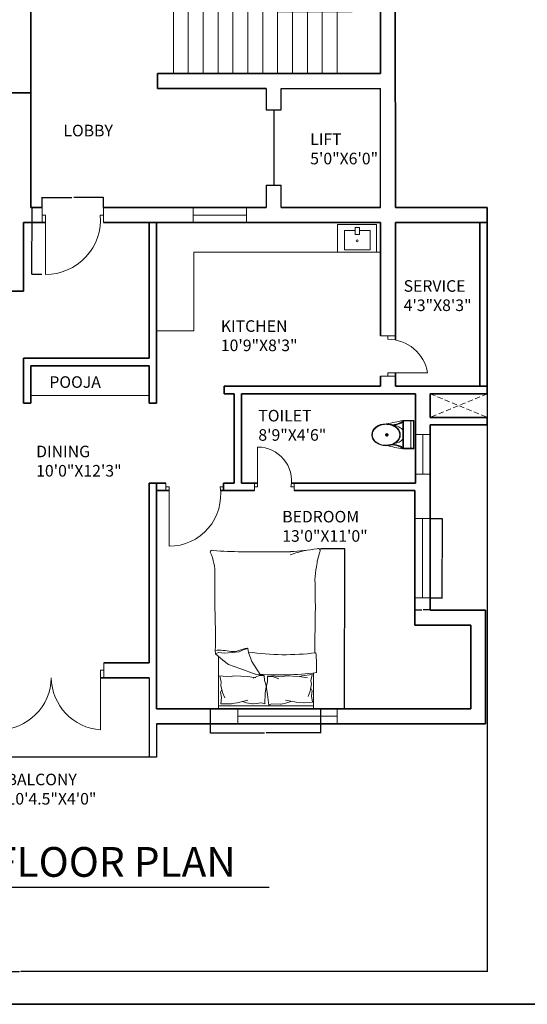
# Model space of a CAD drawing. Units: inches. Extents: x 2296 to 3812, y -1531 to 2564.
# Tile 2 of 10: x 2706 to 3013, y 1124 to 1719. Entities that reach past the tile are written whole.
import ezdxf

# ---------------------------------------------------------------- set-up
doc = ezdxf.new("R2010")
doc.units = ezdxf.units.IN
doc.linetypes.add('HIDDEN2', pattern=[4.7625, 3.175, -1.5875])
for name, color, linetype, lineweight in [('A-ANNO-DIMS', 2, 'Continuous', 18), ('A-ANNO-TEXT', 7, 'Continuous', 25), ('A-ANNO-TTLB', 7, 'Continuous', 35), ('A-AREA-IDEN', 7, 'Continuous', 18), ('A-DOOR', 3, 'Continuous', 18), ('A-EQPM-ELEV', 7, 'Continuous', 25), ('A-FLOR-CASE', 8, 'Continuous', 18), ('A-FLOR-FIXT', 9, 'Continuous', 18), ('A-FLOR-HRAL', 7, 'Continuous', 25), ('A-FLOR-STRS', 7, 'Continuous', 18), ('A-FURN', 8, 'Continuous', 18), ('A-GLAZ', 4, 'Continuous', 18), ('A-WALL', 7, 'Continuous', 35), ('A-WALL-HIDN', 8, 'HIDDEN2', 18)]:
    doc.layers.add(name, color=color, linetype=linetype, lineweight=lineweight)
doc.styles.get("Standard").update_dxf_attribs({"font": 'arial.ttf'})
doc.dimstyles.get("Standard").update_dxf_attribs({"dimtxt": 0.18, "dimasz": 0.18, "dimexe": 0.18, "dimexo": 0.0625, "dimgap": 0.09, "dimtad": 0, "dimtih": 1, "dimtoh": 1, "dimdec": 4, "dimzin": 0, "dimdsep": 46, "dimtxsty": 'Standard', "dimcen": 0.09, "dimadec": 0, "dimazin": 0, "dimtfac": 1, "dimtdec": 4, "dimtofl": 0, "dimtmove": 0, "dimatfit": 3, "dimfxl": 1, "dimtolj": 1, "dimtzin": 0, "dimarcsym": 0})

# ---------------------------------------------------------------- blocks, each defined once
blk = doc.blocks.new('A$C31115884')
for p, q in [((283, 498), (223, 498)), ((258, 466), (258, 523)), ((0, 200), (0, 0)), ((520, 200), (0, 200)), ((10, 190), (10, 10)), ((510, 190), (10, 190)), ((510, 10), (510, 190)), ((520, 0), (520, 200)), ((510, 54), (0, 54)), ((10, 10), (510, 10)), ((0, 0), (520, 0))]:
    blk.add_line(p, q)
blk.add_circle((256, 496), 23.6)
for centre, radius, start, end in [((2778, -205), 2807, 165.4549, 171.7133), ((-295, 403), 365, 324.2091, 9.3499), ((-295, 403), 375, 324.2091, 9.3499), ((139, 406), 293, 315.8436, 2.6563), ((806, 403), 375, 179.2036, 215.7909), ((806, 403), 365, 170.6501, 215.7909), ((3237, 905), 2807, 188.2867, 194.5451), ((384, 406), 293, 190.2774, 224.1564)]:
    blk.add_arc(centre, radius, start, end)
blk.add_ellipse((256, 510), major_axis=(0, -261), ratio=0.772727)
blk.add_open_spline([(256, 259), (263, 259), (270, 260), (288, 262), (299, 265), (320, 273), (330, 278), (350, 291), (360, 299), (378, 316), (386, 326), (402, 347), (409, 358), (421, 383), (427, 395), (436, 422), (440, 436), (445, 465), (447, 480), (448, 509), (448, 524), (445, 553), (443, 568), (436, 596), (432, 610), (422, 636), (416, 649), (402, 672), (395, 683), (379, 703), (370, 712), (351, 728), (341, 735), (321, 746), (310, 751), (289, 757), (278, 759), (256, 761), (245, 761), (223, 757), (212, 754), (191, 746), (181, 741), (161, 728), (151, 720), (133, 703), (125, 693), (110, 672), (103, 660), (90, 636), (85, 623), (76, 596), (72, 582), (67, 553), (66, 538), (64, 509), (65, 494), (68, 465), (70, 450), (77, 422), (81, 408), (91, 382), (97, 370), (111, 346), (118, 335), (135, 316), (144, 307), (162, 291), (172, 284), (193, 273), (203, 269), (225, 262), (236, 260), (250, 259), (253, 259), (256, 259)], degree=3, knots=[0, 0, 0, 0, 0.110105, 0.110105, 0.285049, 0.285049, 0.459994, 0.459994, 0.634938, 0.634938, 0.809882, 0.809882, 0.984827, 0.984827, 1.159771, 1.159771, 1.334715, 1.334715, 1.50966, 1.50966, 1.684604, 1.684604, 1.859549, 1.859549, 2.034493, 2.034493, 2.209437, 2.209437, 2.384382, 2.384382, 2.559326, 2.559326, 2.73427, 2.73427, 2.909215, 2.909215, 3.084159, 3.084159, 3.259103, 3.259103, 3.434048, 3.434048, 3.608992, 3.608992, 3.783936, 3.783936, 3.958881, 3.958881, 4.133825, 4.133825, 4.30877, 4.30877, 4.483714, 4.483714, 4.658658, 4.658658, 4.833603, 4.833603, 5.008547, 5.008547, 5.183491, 5.183491, 5.358436, 5.358436, 5.53338, 5.53338, 5.708324, 5.708324, 5.883269, 5.883269, 6.058213, 6.058213, 6.233158, 6.233158, 6.283185, 6.283185, 6.283185, 6.283185])
blk = doc.blocks.new('DOOR-ENTRY-36-S')
for p, q in [((0, 40.5), (0, 31.5)), ((0, 31.5), (0, 36)), ((0, 36), (2, 36)), ((2, 36), (2, 0)), ((37.2, 36), (35.2, 36)), ((37.2, 40.5), (37.2, 31.5)), ((37.2, 31.5), (37.2, 36))]:
    blk.add_line(p, q)
blk.add_arc((2, 33.31), 33.31, 270, 4.6283)
blk = doc.blocks.new('DOOR-BEDROOM-36-SE')
for p, q in [((0, 38.25), (0, 33.75)), ((0, 33.75), (0, 36)), ((0, 36), (2, 36)), ((2, 36), (2, 0)), ((34.88, 36), (32.88, 36))]:
    blk.add_line(p, q)
blk.add_arc((2, 31.24), 31.24, 270, 8.75969)
blk = doc.blocks.new('DOOR-BATH-24-SE')
for p, q in [((2, 2.25), (2, 26.25)), ((0, 4.5), (0, 0)), ((0, 0), (0, 2.25)), ((0, 2.25), (2, 2.25)), ((24.15, 2.25), (22.15, 2.25)), ((24.15, 4.5), (24.15, 0)), ((24.15, 0), (24.15, 2.25))]:
    blk.add_line(p, q)
blk.add_arc((2, 5.79), 20.46, 350.03773, 90)
blk = doc.blocks.new('DOOR-BALCONY-PAIR-S')
for p, q in [((0, 40.5), (0, 31.5)), ((0, 31.5), (0, 36)), ((0, 36), (2, 36)), ((2, 36), (2, 0)), ((65.68, 36), (63.68, 36)), ((63.68, 36), (63.68, 0)), ((65.68, 40.5), (65.68, 31.5)), ((65.68, 31.5), (65.68, 36))]:
    blk.add_line(p, q)
for centre, radius, start, end in [((2, 31.87), 31.87, 270, 359.32793), ((65.8, 31.86), 31.93, 180.64039, 266.18908)]:
    blk.add_arc(centre, radius, start, end)
blk = doc.blocks.new('DOOR-SERVICE-24-SE')
for p, q in [((9, 24.24), (0, 24.24)), ((0, 24.24), (4.5, 24.24)), ((4.5, 24.24), (4.5, 22.24)), ((9, 0), (0, 0)), ((0, 0), (4.5, 0)), ((4.5, 0), (4.5, 2)), ((4.5, 2), (28.5, 2))]:
    blk.add_line(p, q)
blk.add_arc((4.5, -2.11), 24.35, 9.71884, 90)
blk = doc.blocks.new('WIN-24-BATH')
for p, q in [((4.5, 24), (0, 24)), ((0, 24), (9, 24)), ((4.5, 0), (4.5, 24)), ((0, 0), (9, 0)), ((9, 0), (4.5, 0))]:
    blk.add_line(p, q)
blk = doc.blocks.new('WIN-48-BEDROOM-SE')
for p, q in [((4.71, 48), (0, 48)), ((0, 48), (9.41, 48)), ((4.71, 0), (4.71, 48)), ((0, 0), (9.41, 0)), ((9.41, 0), (4.71, 0))]:
    blk.add_line(p, q)
blk = doc.blocks.new('WIN-60-SILL')
for p, q in [((0, 9), (0, 0)), ((60, 4.5), (60, 9)), ((60, 9), (60, 0)), ((0, 0), (0, 4.5)), ((0, 4.5), (60, 4.5))]:
    blk.add_line(p, q)
blk = doc.blocks.new('WIN-32-KITCHEN')
for p, q in [((0, 9), (0, 0)), ((32.18, 4.5), (32.18, 9)), ((32.18, 9), (32.18, 0)), ((0, 0), (0, 4.5)), ((0, 4.5), (32.18, 4.5))]:
    blk.add_line(p, q)
blk = doc.blocks.new('BED-DOUBLE')
for p, q in [((48.49, 95), (18.98, 95)), ((22.83, 36.42), (19.86, 35.68)), ((23.21, 34.01), (22.83, 36.42)), ((3.07, 35.36), (3.17, 33.26, 4.64)), ((5.01, 34.01), (3.17, 33.26)), ((3.17, 33.26), (7.61, 29.37)), ((8.72, 33.63), (5.01, 34.01)), ((5.09, 0), (5.09, 31.9)), ((13.37, 34.01), (8.72, 33.63)), ((17.45, 34.56), (13.37, 34.01)), ((19.86, 35.68), (17.45, 34.56)), ((25.25, 28.62), (23.21, 34.01)), ((7.61, 29.37), (11.14, 26.77)), ((11.14, 26.77), (17.82, 24.36)), ((17.82, 24.36), (27.82, 20.84)), ((30.27, 20.84), (25.25, 28.62)), ((11.92, 19.38), (5.77, 19.87)), ((5.77, 19.87), (6.7, 16.11)), ((14.27, 20.05), (11.92, 19.38)), ((22.67, 19.54), (14.27, 20.05)), ((27.51, 18.74), (22.67, 19.54)), ((29.68, 20.07), (26, 18.53)), ((32.62, 20.25), (29.68, 20.07)), ((32.82, 17.04), (32.62, 20.25)), ((34.71, 16.28), (34.71, 19.5)), ((34.71, 19.5), (37.65, 19.5)), ((43.31, 19.38), (37.16, 19.87)), ((37.65, 19.5), (41.42, 18.19)), ((45.66, 20.05), (43.31, 19.38)), ((54.06, 19.54), (45.66, 20.05)), ((54.06, 19.54), (55.42, 19.92)), ((58.9, 18.74), (54.06, 19.54)), ((55.42, 19.92), (61.53, 20.79)), ((61.53, 20.79), (60.84, 16.98)), ((62.38, 21.71), (62.38, 0)), ((6.7, 16.11), (6.47, 14.18)), ((6.47, 14.18), (7.43, 9.9)), ((33.66, 14.84), (32.82, 17.04)), ((33.3, 9.43), (33.75, 13.28)), ((33.75, 13.28), (33.66, 14.84)), ((34.01, 14.03), (34.71, 16.28)), ((34.01, 12.47), (34.01, 14.03)), ((34.71, 8.66), (34.01, 12.47)), ((61.19, 15.07), (60.49, 10.74)), ((60.84, 16.98), (61.19, 15.07)), ((61.71, 10.91), (61.01, 12.12)), ((6.21, 10), (6.83, 11.25)), ((6.93, 6.92), (6.21, 10)), ((6.47, 3.07), (6.93, 6.92)), ((7.43, 9.9), (8.85, 6.69)), ((33.01, 2.99), (33.3, 9.43)), ((35.4, 2.24), (34.71, 8.66)), ((60.49, 10.74), (59.28, 7.44)), ((61.19, 7.79), (61.71, 10.91)), ((61.88, 3.98), (61.19, 7.79)), ((62.38, 1.84), (5.09, 1.84)), ((62.38, 0), (5.09, 0)), ((6.47, 3.07), (12.95, 2.95)), ((11.75, 3.05), (16.3, 3.68)), ((12.95, 2.95), (11.75, 3.05)), ((16.3, 3.68), (22.8, 5.3)), ((19.55, 4.4), (22.03, 3.69)), ((22.03, 3.69), (25.54, 3.04)), ((25.54, 3.04), (25.93, 3.07)), ((25.93, 3.07), (31.24, 3.57)), ((31.24, 3.57), (33.01, 2.99)), ((37.13, 2.94), (35.4, 2.24)), ((42.46, 2.76), (37.13, 2.94)), ((42.85, 2.76), (42.46, 2.76)), ((46.31, 3.63), (42.85, 2.76)), ((52.03, 3.98), (45.45, 5.19)), ((48.74, 4.5), (46.31, 3.63)), ((56.62, 3.63), (52.03, 3.98)), ((56.74, 3.61), (56.62, 3.63)), ((61.87, 4), (56.74, 3.61))]:
    blk.add_line(p, q)
for centre, radius, start, end in [((1.32, 94.55), 1.32, 62.65876, 176.02002), ((17.21, 254.49), 159.5, 264.4998, 270.63509), ((87.19, -28.43), 127.63, 103.38322, 107.70533), ((40.86, 240.78), 145.97, 272.99578, 279.40907), ((65.24, 95.57), 1.31, 326.17358, 113.47814), ((-24.75, 82.32), 27.65, 357.47136, 26.46809), ((92.52, 84.25), 28.25, 157.97508, 176.652), ((98.8, 77.34), 35.53, 166.06484, 178.91125), ((5471.89, 81.31), 5469.02, 180.00217, 180.28689), ((-514.68, 60.68), 578.22, 358.22771, 1.71854), ((-151.96, 43.54), 155.25, 356.97912, 3.83645), ((267.13, 37.37), 203.94, 178.4762, 181.00819), ((29.2, 1.78), 35.55, 100.66171, 109.88058), ((22.63, 36.49), 0.221, 340.24637, 91.13765), ((5.01, -7.98), 43.38, 79.87628, 92.56571), ((14.11, 42.04), 7.46, 258.6608, 293.73842), ((45.26, 187.4), 154.68, 261.78449, 276.90062), ((-35.55, 24.09), 99.87, 358.72178, 5.60397), ((40.94, 218.26), 197.77, 266.08655, 276.78213)]:
    blk.add_arc(centre, radius, start, end)
blk = doc.blocks.new('SINK-KITCHEN')
for points in [[(0, 16.77), (23.71, 16.77), (23.71, 0), (0, 0)], [(10.76, 14.92), (13.44, 14.92), (13.44, 10.63), (10.76, 10.63)]]:
    blk.add_lwpolyline(points, close=True)
blk.add_lwpolyline([(13.44, 13.06), (19.73, 13.06), (19.73, 1.48), (4.23, 1.48), (4.23, 13.06), (10.76, 13.06)])
blk.add_circle((11.97, 6.87), 0.556)
blk = doc.blocks.new('STAIR-DOGLEG')
for p, q in [((20.27, 0), (20.27, 152.06)), ((29.27, 0), (29.27, 152.06)), ((38.27, 0), (38.27, 152.06)), ((47.27, 0), (47.27, 152.06)), ((56.27, 0), (56.27, 152.06)), ((65.27, 0), (65.27, 152.06)), ((74.27, 0), (74.27, 152.06)), ((83.27, 0), (83.27, 152.06)), ((92.27, 0), (92.27, 152.06)), ((101.27, 0), (101.27, 152.06)), ((110.27, 0), (110.27, 152.06)), ((119.27, 0), (119.27, 152.06)), ((0, 107.85), (128.27, 107.85)), ((128.27, 107.85), (128.27, 37.4)), ((20.27, 76.03), (119.27, 76.03)), ((128.27, 37.4), (83.27, 37.4))]:
    blk.add_line(p, q)
blk = doc.blocks.new('COUNTER-KITCHEN-S')
for p, q in [((22.51, 0), (22.51, 47.52)), ((22.51, 47.52), (135.34, 47.52)), ((0, 0), (0, 0)), ((0, 0), (22.51, 0))]:
    blk.add_line(p, q)
blk = doc.blocks.new('LIFT-SHAFT-60x72')
for p, q in [((0, 72), (0, 59.12)), ((9, 72), (69, 72)), ((9, 59.12), (9, 72)), ((69, 0), (69, 72)), ((0, 59.12), (9, 59.12)), ((4.5, 59.12), (4.5, 13.58)), ((0, 13.58), (9, 13.58)), ((0, 13.58), (0, 0)), ((9, 0), (9, 13.58)), ((69, 0), (9, 0)), ((9, 0), (69, 0))]:
    blk.add_line(p, q)
blk = doc.blocks.new('*D43')
at = {"layer": 'A-ANNO-DIMS', "color": 0, "lineweight": -2, "transparency": 16777216}
for p, q in [((2888.22, 1399.6), (2902.88, 1399.6)), ((2902.7, 1399.42), (2902.7, 1351.28)), ((2902.7, 1302.78), (2902.7, 1350.92)), ((2888.22, 1302.6), (2902.88, 1302.6))]:
    blk.add_line(p, q, dxfattribs=at)
at = {"layer": 'A-ANNO-DIMS', "color": 0, "transparency": 16777216}
for points in [[(2902.67, 1399.42), (2902.73, 1399.42), (2902.7, 1399.6)], [(2902.67, 1302.78), (2902.73, 1302.78), (2902.7, 1302.6)]]:
    blk.add_solid(points, dxfattribs=at)
at = {"layer": 'Defpoints', "color": 0, "transparency": 16777216}
for p in [(2888.15, 1399.6), (2902.7, 1399.6), (2888.15, 1302.6)]:
    blk.add_point(p, dxfattribs=at)
at = {"layer": 'A-ANNO-DIMS', "color": 0, "transparency": 16777216, "insert": (2902.7, 1351.1), "char_height": 0.18, "attachment_point": 5}
blk.add_mtext('\\A1;BED 97 TYP.', dxfattribs=at)
blk = doc.blocks.new('*D44')
at = {"layer": 'A-ANNO-DIMS', "color": 0, "lineweight": -2, "transparency": 16777216}
for p, q in [((2821.5, 1302.54), (2821.5, 1287.87)), ((2888.15, 1302.54), (2888.15, 1287.87)), ((2821.68, 1288.05), (2854.3, 1288.05)), ((2887.97, 1288.05), (2855.36, 1288.05))]:
    blk.add_line(p, q, dxfattribs=at)
at = {"layer": 'A-ANNO-DIMS', "color": 0, "transparency": 16777216}
for points in [[(2821.68, 1288.08), (2821.68, 1288.02), (2821.5, 1288.05)], [(2887.97, 1288.08), (2887.97, 1288.02), (2888.15, 1288.05)]]:
    blk.add_solid(points, dxfattribs=at)
at = {"layer": 'Defpoints', "color": 0, "transparency": 16777216}
for p in [(2821.5, 1302.6), (2888.15, 1302.6), (2888.15, 1288.05)]:
    blk.add_point(p, dxfattribs=at)
at = {"layer": 'A-ANNO-DIMS', "color": 0, "transparency": 16777216, "insert": (2854.83, 1288.05), "char_height": 0.18, "attachment_point": 5}
blk.add_mtext('\\A1;67 TYP.', dxfattribs=at)
blk = doc.blocks.new('*D77')
at = {"layer": 'A-ANNO-DIMS', "color": 0, "lineweight": -2, "transparency": 16777216}
for p, q in [((2719.83, 1605.6), (2713.64, 1605.6)), ((2713.82, 1605.42), (2713.82, 1585.53)), ((2713.82, 1565.28), (2713.82, 1585.17)), ((2719.83, 1565.1), (2713.64, 1565.1))]:
    blk.add_line(p, q, dxfattribs=at)
at = {"layer": 'A-ANNO-DIMS', "color": 0, "transparency": 16777216}
for points in [[(2713.79, 1605.42), (2713.85, 1605.42), (2713.82, 1605.6)], [(2713.79, 1565.28), (2713.85, 1565.28), (2713.82, 1565.1)]]:
    blk.add_solid(points, dxfattribs=at)
at = {"layer": 'Defpoints', "color": 0, "transparency": 16777216}
for p in [(2713.82, 1605.6), (2719.89, 1605.6), (2719.89, 1565.1)]:
    blk.add_point(p, dxfattribs=at)
at = {"layer": 'A-ANNO-DIMS', "color": 0, "transparency": 16777216, "insert": (2713.82, 1585.35), "char_height": 0.18, "attachment_point": 5}
blk.add_mtext('\\A1;ENTRY DOOR 41 TYP.', dxfattribs=at)
blk = doc.blocks.new('*D78')
at = {"layer": 'A-ANNO-DIMS', "color": 0, "lineweight": -2, "transparency": 16777216}
for p, q in [((2719.89, 1605.66), (2719.89, 1611.86)), ((2720.07, 1611.68), (2737.97, 1611.68)), ((2756.92, 1611.68), (2739.02, 1611.68)), ((2757.1, 1605.66), (2757.1, 1611.86))]:
    blk.add_line(p, q, dxfattribs=at)
at = {"layer": 'A-ANNO-DIMS', "color": 0, "transparency": 16777216}
for points in [[(2720.07, 1611.71), (2720.07, 1611.65), (2719.89, 1611.68)], [(2756.92, 1611.71), (2756.92, 1611.65), (2757.1, 1611.68)]]:
    blk.add_solid(points, dxfattribs=at)
at = {"layer": 'Defpoints', "color": 0, "transparency": 16777216}
for p in [(2757.1, 1611.68), (2719.89, 1605.6), (2757.1, 1605.6)]:
    blk.add_point(p, dxfattribs=at)
at = {"layer": 'A-ANNO-DIMS', "color": 0, "transparency": 16777216, "insert": (2738.5, 1611.68), "char_height": 0.18, "attachment_point": 5}
blk.add_mtext('\\A1;37 TYP.', dxfattribs=at)
blk = doc.blocks.new('*D105')
at = {"layer": 'A-ANNO-DIMS', "color": 0, "lineweight": -2, "transparency": 16777216}
for p, q in [((2954.54, 1417.69), (2961.86, 1417.69)), ((2961.68, 1417.51), (2961.68, 1393.87)), ((2961.68, 1369.87), (2961.68, 1393.51)), ((2954.54, 1369.69), (2961.86, 1369.69))]:
    blk.add_line(p, q, dxfattribs=at)
at = {"layer": 'A-ANNO-DIMS', "color": 0, "transparency": 16777216}
for points in [[(2961.65, 1417.51), (2961.71, 1417.51), (2961.68, 1417.69)], [(2961.65, 1369.87), (2961.71, 1369.87), (2961.68, 1369.69)]]:
    blk.add_solid(points, dxfattribs=at)
at = {"layer": 'Defpoints', "color": 0, "transparency": 16777216}
for p in [(2954.48, 1417.69), (2961.68, 1417.69), (2954.48, 1369.69)]:
    blk.add_point(p, dxfattribs=at)
at = {"layer": 'A-ANNO-DIMS', "color": 0, "transparency": 16777216, "insert": (2961.68, 1393.69), "char_height": 0.18, "attachment_point": 5}
blk.add_mtext('\\A1;WINDOW 48 TYP.', dxfattribs=at)
blk = doc.blocks.new('*D106')
at = {"layer": 'A-ANNO-DIMS', "color": 0, "lineweight": -2, "transparency": 16777216}
for p, q in [((2945.07, 1369.63), (2945.07, 1362.31)), ((2954.48, 1369.63), (2954.48, 1362.31)), ((2945.25, 1362.49), (2949.32, 1362.49)), ((2954.3, 1362.49), (2950.23, 1362.49))]:
    blk.add_line(p, q, dxfattribs=at)
at = {"layer": 'A-ANNO-DIMS', "color": 0, "transparency": 16777216}
for points in [[(2945.25, 1362.52), (2945.25, 1362.46), (2945.07, 1362.49)], [(2954.3, 1362.52), (2954.3, 1362.46), (2954.48, 1362.49)]]:
    blk.add_solid(points, dxfattribs=at)
at = {"layer": 'Defpoints', "color": 0, "transparency": 16777216}
for p in [(2945.07, 1369.69), (2954.48, 1369.69), (2954.48, 1362.49)]:
    blk.add_point(p, dxfattribs=at)
at = {"layer": 'A-ANNO-DIMS', "color": 0, "transparency": 16777216, "insert": (2949.77, 1362.49), "char_height": 0.18, "attachment_point": 5}
blk.add_mtext('\\A1;9 TYP.', dxfattribs=at)
blk = doc.blocks.new('*D127')
at = {"layer": 'A-ANNO-DIMS', "color": 0, "lineweight": -2, "transparency": 16777216}
for p, q in [((2988.9, 1498.34), (2988.9, 1143.72)), ((2424.57, 1427.77), (2424.57, 1143.72)), ((2424.75, 1143.9), (2706.34, 1143.9)), ((2988.72, 1143.9), (2707.13, 1143.9))]:
    blk.add_line(p, q, dxfattribs=at)
at = {"layer": 'A-ANNO-DIMS', "color": 0, "transparency": 16777216}
for points in [[(2424.75, 1143.93), (2424.75, 1143.87), (2424.57, 1143.9)], [(2988.72, 1143.93), (2988.72, 1143.87), (2988.9, 1143.9)]]:
    blk.add_solid(points, dxfattribs=at)
at = {"layer": 'Defpoints', "color": 0, "transparency": 16777216}
for p in [(2988.9, 1498.4), (2424.57, 1427.84), (2988.9, 1143.9)]:
    blk.add_point(p, dxfattribs=at)
at = {"layer": 'A-ANNO-DIMS', "color": 0, "transparency": 16777216, "insert": (2706.74, 1143.9), "char_height": 0.18, "attachment_point": 5}
blk.add_mtext('\\A1;564.3', dxfattribs=at)

msp = doc.modelspace()

# ---------------------------------------------------------------- linework, layer by layer
at = {"layer": 'A-ANNO-TEXT'}
msp.add_line((2618.3678, 1194.7471), (2857.1248, 1194.7471), dxfattribs=at)
at = {"layer": 'A-ANNO-TTLB'}
msp.add_lwpolyline([(2296.1257, 2564.2989), (3812.4193, 2564.2989), (3812.4193, 1124.0028), (2296.1257, 1124.0028)], close=True, dxfattribs=at)
at = {"layer": 'A-FLOR-CASE'}
msp.add_line((2713.1222, 1492.0877), (2784.5693, 1492.0877), dxfattribs=at)
at = {"layer": 'A-FLOR-HRAL'}
for p, q in [((2784.5693, 1321.434), (2784.5693, 1273.434)), ((2784.5693, 1321.434), (2784.5693, 1302.6012)), ((2784.5693, 1302.6012), (2784.5693, 1273.434)), ((2789.0693, 1293.6012), (2789.0693, 1273.434)), ((2784.5693, 1273.434), (2670.7523, 1273.434)), ((2789.0693, 1273.434), (2784.5693, 1273.434))]:
    msp.add_line(p, q, dxfattribs=at)
at = {"layer": 'A-WALL'}
for p, q in [((2924.405, 1686.6012), (2924.405, 1838.6578)), ((2933.0693, 1838.6578), (2933.405, 1605.6012)), ((2713.1754, 1780.1578), (2713.1754, 1674.9485)), ((2855.405, 1686.6012), (2789.6622, 1686.6012)), ((2789.6622, 1686.6012), (2789.6622, 1677.6012)), ((2864.405, 1686.6012), (2855.405, 1686.6012)), ((2924.405, 1686.6012), (2864.405, 1686.6012)), ((2638.4, 1674.9485), (2713.1754, 1674.9485)), ((2713.1754, 1674.9485), (2713.1754, 1605.6012)), ((2789.6622, 1677.6012), (2855.405, 1677.6012)), ((2713.1754, 1605.6012), (2719.8939, 1605.6012)), ((2757.0973, 1605.6012), (2855.405, 1605.6012)), ((2933.405, 1605.6012), (2988.905, 1605.6012)), ((2988.905, 1596.6012), (2988.905, 1605.6012)), ((2713.1754, 1596.6012), (2708.6222, 1596.6012)), ((2708.6222, 1596.6012), (2708.6222, 1555.1578)), ((2713.1754, 1596.6012), (2721.8939, 1596.6012)), ((2757.0973, 1596.6012), (2924.405, 1596.6012)), ((2784.5693, 1596.6012), (2784.5693, 1514.5213)), ((2789.0693, 1596.6012), (2789.0693, 1487.3045)), ((2789.0693, 1596.6012), (2918.0693, 1596.6012)), ((2924.405, 1527.9833), (2924.405, 1596.6012)), ((2933.405, 1596.6012), (2933.405, 1525.5639)), ((2933.405, 1596.6012), (2984.405, 1596.6012)), ((2933.405, 1596.6012), (2984.405, 1596.6012)), ((2984.405, 1596.6012), (2984.405, 1497.6012)), ((2984.405, 1596.6012), (2988.905, 1596.6012)), ((2988.905, 1596.6012), (2988.905, 1498.4048)), ((2708.6222, 1555.1578), (2633.9, 1555.1578)), ((2924.405, 1538.1945), (2924.405, 1538.1945)), ((2708.6222, 1514.5213), (2708.6222, 1487.3045)), ((2708.6222, 1487.3045), (2708.6222, 1514.5213)), ((2708.6222, 1514.5213), (2784.5693, 1514.5213)), ((2784.5693, 1510.0213), (2713.1222, 1510.0213)), ((2713.1222, 1510.0213), (2713.1222, 1487.3045)), ((2784.5693, 1510.0213), (2784.5693, 1487.3045)), ((2924.405, 1497.6012), (2924.405, 1503.7443)), ((2933.405, 1505.7443), (2933.405, 1497.6012)), ((2829.8641, 1497.6012), (2924.405, 1497.6012)), ((2829.8641, 1497.6012), (2829.8641, 1493.1012)), ((2933.405, 1497.6012), (2984.405, 1497.6012)), ((2984.405, 1497.6012), (2988.905, 1497.6012)), ((2988.905, 1493.1012), (2988.905, 1498.4048)), ((2829.8641, 1493.1012), (2835.9796, 1493.1012)), ((2835.9796, 1439.1012), (2835.9796, 1493.1012)), ((2945.4796, 1493.1012), (2840.4796, 1493.1012)), ((2840.4796, 1493.1012), (2840.4796, 1439.1012)), ((2840.4796, 1493.1012), (2945.4796, 1493.1012)), ((2945.4796, 1439.1012), (2945.4796, 1493.1012)), ((2954.4796, 1493.1012), (2954.4796, 1478.7391)), ((2954.4796, 1493.1012), (2984.405, 1493.1012)), ((2984.405, 1493.1012), (2988.905, 1493.1012)), ((2713.1222, 1487.3045), (2708.6222, 1487.3045)), ((2789.0693, 1487.3045), (2784.5693, 1487.3045)), ((2988.905, 1478.7391), (2954.4796, 1478.7391)), ((2988.905, 1474.2391), (2988.905, 1478.7391)), ((2954.4796, 1474.2391), (2988.905, 1474.2391)), ((2954.4796, 1474.2391), (2954.4796, 1439.1012)), ((2794.6251, 1439.1012), (2784.5693, 1439.1012)), ((2784.5693, 1439.1012), (2784.5693, 1330.434)), ((2789.0693, 1439.1012), (2789.0693, 1302.6012)), ((2796.6251, 1434.6012), (2789.0693, 1434.6012)), ((2829.5028, 1434.6012), (2827.7664, 1434.6012)), ((2829.5028, 1439.1012), (2835.9796, 1439.1012)), ((2829.5028, 1439.1012), (2829.5028, 1434.6012)), ((2829.5028, 1434.6012), (2848.1807, 1434.6012)), ((2840.4796, 1434.6012), (2835.9796, 1434.6012)), ((2840.4796, 1439.1012), (2850.1807, 1439.1012)), ((2870.6004, 1439.1012), (2945.4796, 1439.1012)), ((2872.3326, 1434.6012), (2945.0693, 1434.6012)), ((2945.0693, 1353.1926), (2945.0693, 1434.6012)), ((2954.4796, 1439.1012), (2954.4796, 1362.1926)), ((2954.4796, 1362.1926), (2987.9477, 1362.1926)), ((2987.9477, 1362.1926), (2978.9477, 1362.1926)), ((2987.9477, 1293.6012), (2987.9477, 1362.1926)), ((2978.9477, 1353.1926), (2945.0693, 1353.1926)), ((2978.9477, 1353.1926), (2978.9477, 1302.6012)), ((2784.5693, 1330.434), (2757.3002, 1330.434)), ((2755.3002, 1321.434), (2784.5693, 1321.434)), ((2789.0693, 1302.6012), (2945.0693, 1302.6012)), ((2789.0693, 1302.6012), (2978.9477, 1302.6012)), ((2789.0693, 1293.6012), (2984.405, 1293.6012)), ((2984.405, 1293.6012), (2987.9477, 1293.6012))]:
    msp.add_line(p, q, dxfattribs=at)
at = {"layer": 'A-WALL-HIDN'}
for p, q in [((2988.905, 1493.1012), (2954.4796, 1478.7391)), ((2954.4796, 1493.1012), (2988.905, 1478.7391))]:
    msp.add_line(p, q, dxfattribs=at)

# ---------------------------------------------------------------- block references
at = {"layer": 'A-DOOR'}
for name, p in [('DOOR-ENTRY-36-S', (2719.894, 1565.101)), ('DOOR-SERVICE-24-SE', (2924.405, 1503.744)), ('DOOR-BATH-24-SE', (2848.181, 1434.601)), ('DOOR-BEDROOM-36-SE', (2794.625, 1400.851)), ('DOOR-BALCONY-PAIR-S', (2691.625, 1289.934))]:
    msp.add_blockref(name, p, dxfattribs=at)
at = {"layer": 'A-EQPM-ELEV'}
msp.add_blockref('LIFT-SHAFT-60x72', (2855.405, 1605.601), dxfattribs=at)
at = {"layer": 'A-FLOR-CASE'}
msp.add_blockref('COUNTER-KITCHEN-S', (2789.069, 1531.098), dxfattribs=at)
at = {"layer": 'A-FLOR-FIXT'}
msp.add_blockref('SINK-KITCHEN', (2898.341, 1578.617), dxfattribs=at)
at = {"layer": 'A-FLOR-FIXT', "xscale": 0.0330640103915726, "yscale": 0.0330640103915726, "zscale": 0.0330640103915726, "rotation": 89.99999999999999}
msp.add_blockref('A$C31115884', (2944.6092, 1459.7787), dxfattribs=at)
at = {"layer": 'A-FLOR-STRS'}
msp.add_blockref('STAIR-DOGLEG', (2778.968, 1686.601), dxfattribs=at)
at = {"layer": 'A-FURN'}
msp.add_blockref('BED-DOUBLE', (2821.5008, 1302.601), dxfattribs=at)
at = {"layer": 'A-GLAZ'}
for name, p in [('WIN-32-KITCHEN', (2811.268, 1596.601)), ('WIN-24-BATH', (2945.4794, 1444.5142)), ('WIN-48-BEDROOM-SE', (2945.069, 1369.691)), ('WIN-60-SILL', (2838.135, 1293.601))]:
    msp.add_blockref(name, p, dxfattribs=at)

# ---------------------------------------------------------------- texts
at = {"layer": 'A-ANNO-TEXT', "insert": (2619.7605, 1219.0643), "char_height": 18, "attachment_point": 1}
msp.add_mtext_dynamic_manual_height_columns('FIRST FLOOR PLAN', width=376.570462, gutter_width=12.5, heights=[0], dxfattribs=at)
at = {"layer": 'A-AREA-IDEN', "char_height": 7, "attachment_point": 1}
for s, width, insert in [('LOBBY', 80.041459, (2732.809, 1655.6488)), ('LIFT\\P5\'0"X6\'0"', 51.41973, (2881.9385, 1650.4068)), ('SERVICE\\P4\'3"X8\'3"', 55.005925, (2938.3989, 1561.7174)), ('KITCHEN\\P10\'9"X8\'3"', 84.740182, (2827.9395, 1537.4753)), ('POOJA', 56.385117, (2724.3233, 1503.6221)), ('TOILET\\P8\'9"X4\'6"', 52.406302, (2850.593, 1483.3158)), ('DINING\\P10\'0"X12\'3"', 55.628876, (2716.3407, 1461.6727)), ('BEDROOM\\P13\'0"X11\'0"', 80.045459, (2865.0239, 1422.2672)), ('BALCONY\\P10\'4.5"X4\'0"', 89.884194, (2698.4627, 1263.4036))]:
    msp.add_mtext_dynamic_manual_height_columns(s, width=width, gutter_width=12.5, heights=[0], dxfattribs=dict(at, insert=insert))

# ---------------------------------------------------------------- dimensions: what is measured, and where the dimension line sits
at = {"layer": 'A-ANNO-DIMS'}
for base, p1, p2, picture, middle in [((2757.0973, 1611.6762), (2719.8939, 1605.6012), (2757.0973, 1605.6012), '*D78', (2738.4956, 1611.6762)), ((2954.4796, 1362.4913), (2945.0693, 1369.6913), (2954.4796, 1369.6913), '*D106', (2949.7745, 1362.4913)), ((2888.1526, 1288.0514), (2821.501, 1302.6012), (2888.1526, 1302.6012), '*D44', (2854.8268, 1288.0514))]:
    dim = msp.add_linear_dim(base=base, p1=p1, p2=p2, text='<> TYP.', dimstyle='Standard', override={"dimdec": 0, "dimlfac": 1, "dimrnd": 0, "dimzin": 0, "dimdsep": 46, "dimlunit": 2}, dxfattribs=at)
    dim.commit()
    dim.dimension.update_dxf_attribs({"geometry": picture, "text_midpoint": middle})
for base, p1, p2, text, picture, middle in [((2713.8188818348, 1605.6012203397), (2719.8938818348, 1565.1012203397), (2719.8938818348, 1605.6012203397), 'ENTRY DOOR <> TYP.', '*D77', (2713.8188818348, 1585.3512203397)), ((2961.6796, 1417.6913), (2954.4796, 1369.6913), (2954.4796, 1417.6913), 'WINDOW <> TYP.', '*D105', (2961.6796, 1393.6913)), ((2902.7024, 1399.6), (2888.1526, 1302.6012), (2888.1526, 1399.6), 'BED <> TYP.', '*D43', (2902.7024, 1351.1006))]:
    dim = msp.add_linear_dim(base=base, p1=p1, p2=p2, angle=90, text=text, dimstyle='Standard', override={"dimdec": 0, "dimlfac": 1, "dimrnd": 0, "dimzin": 0, "dimdsep": 46, "dimlunit": 2}, dxfattribs=at)
    dim.commit()
    dim.dimension.update_dxf_attribs({"geometry": picture, "text_midpoint": middle})
dim = msp.add_linear_dim(base=(2988.905, 1143.8971), p1=(2424.5693, 1427.8367), p2=(2988.905, 1498.4048), dimstyle='Standard', override={"dimdec": 1, "dimlfac": 1, "dimrnd": 0, "dimzin": 0, "dimdsep": 46, "dimlunit": 2}, dxfattribs=at)
dim.commit()
dim.dimension.update_dxf_attribs({"geometry": '*D127', "text_midpoint": (2706.7372, 1143.8971)})

doc.saveas('drawing.dxf')
